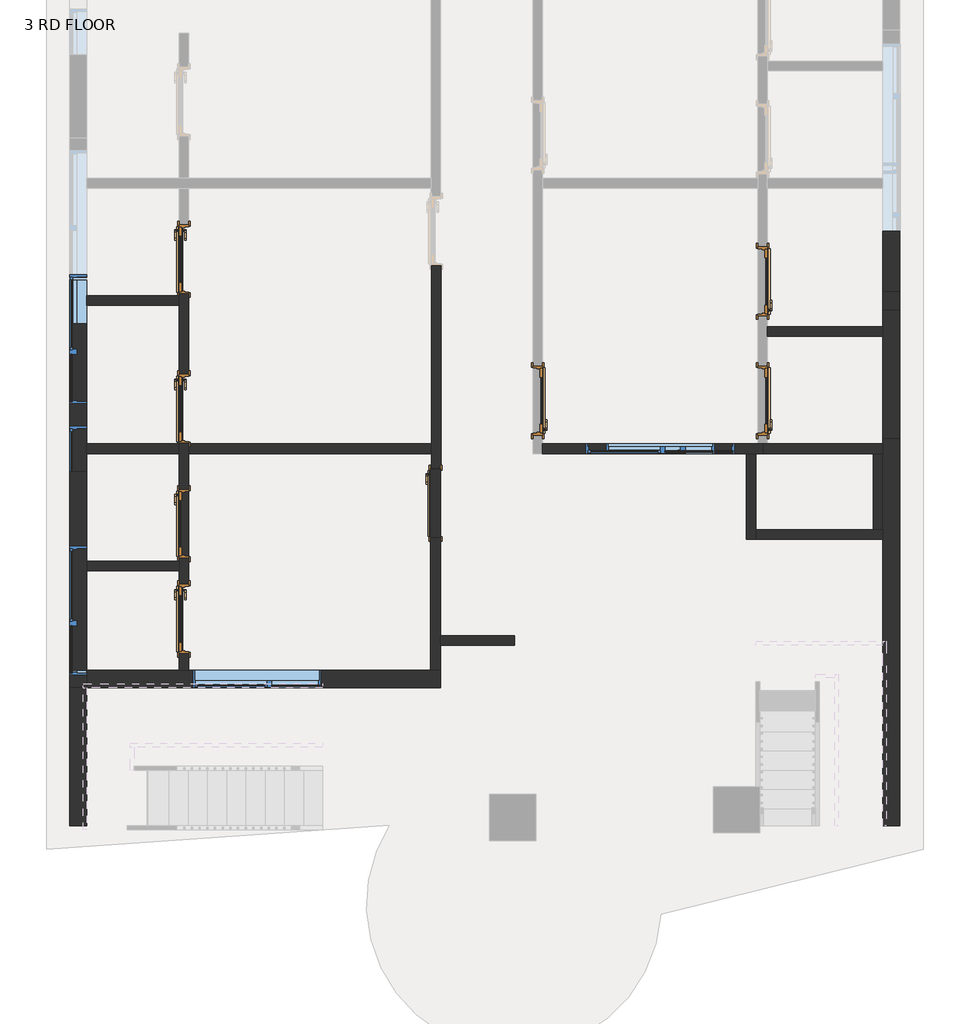
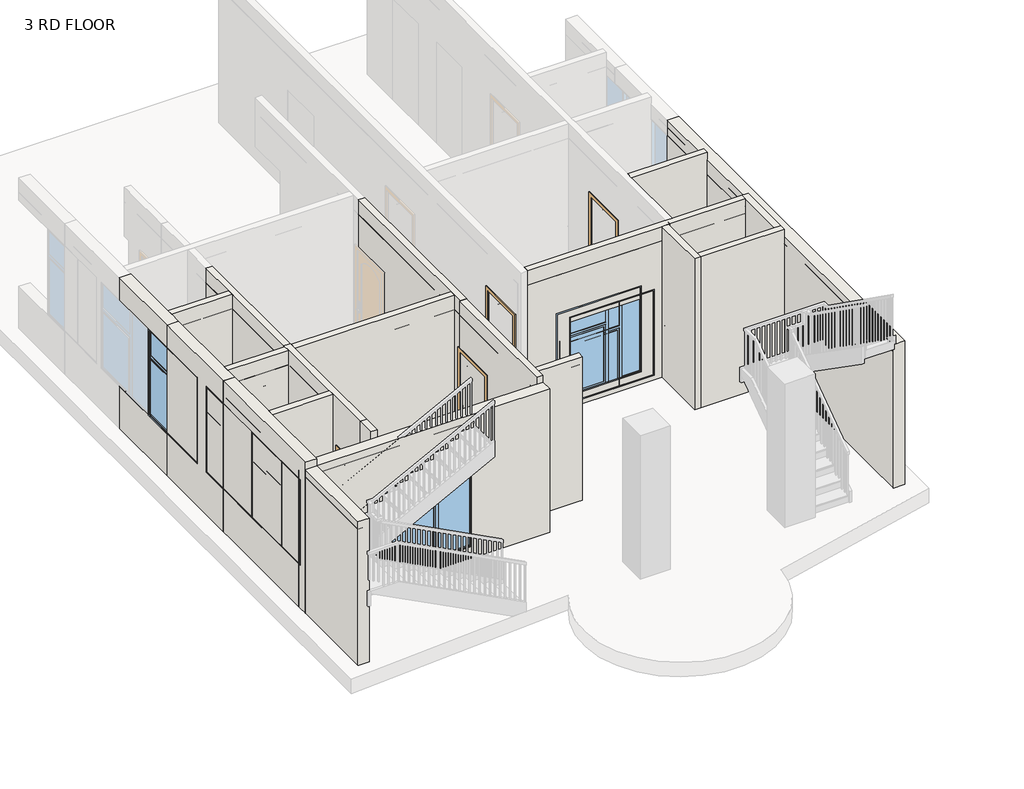
# One storey, part 1 of 5: 41 walls, 8 doors, 7 windows.
# Revit data of these elements (continued)
# Element 55 (IfcWindow, "M_Window-Casement-Double-Sidelight : 1702 x 1829mm")
#   Mark = "76"
#   Window Inset = 0' - 0.62598"
#   Frame Gap 3 = 0' - 1.65041"
#   Frame Gap 2 = 0' - 0.62598"
#   Phase Created = New Construction
#   Materials on its faces: "Metal - Aluminum", "Glass"
# Element 56 (IfcWindow, "M_Window-Casement-Double-Sidelight : 1702 x 1829mm")
#   Mark = "103"
#   Window Inset = 0' - 0.62598"
#   Frame Gap 3 = 0' - 1.65041"
#   Frame Gap 2 = 0' - 0.62598"
#   Phase Created = New Construction
#   Materials on its faces: "Metal - Aluminum", "Glass"
# Materials
#   "Cherry": class "Wood", colour RGB 226 177 128, transparency 0, Description = "Prunus Serotina", Cost = 0
#   "Glass": class "Glass", colour RGB 0 128 192, transparency 0.75, Description = "Soda Lime Glass", Cost = 0
#   "Aluminum": class "Metal", colour RGB 247 247 247, transparency 0, Description = "Aluminum 6061", Cost = 0
#   "Metal - Aluminum": class "Metal", colour RGB 247 247 247, transparency 0
#   "Default Wall": colour RGB 128 128 128, transparency 0, Cost = 0
